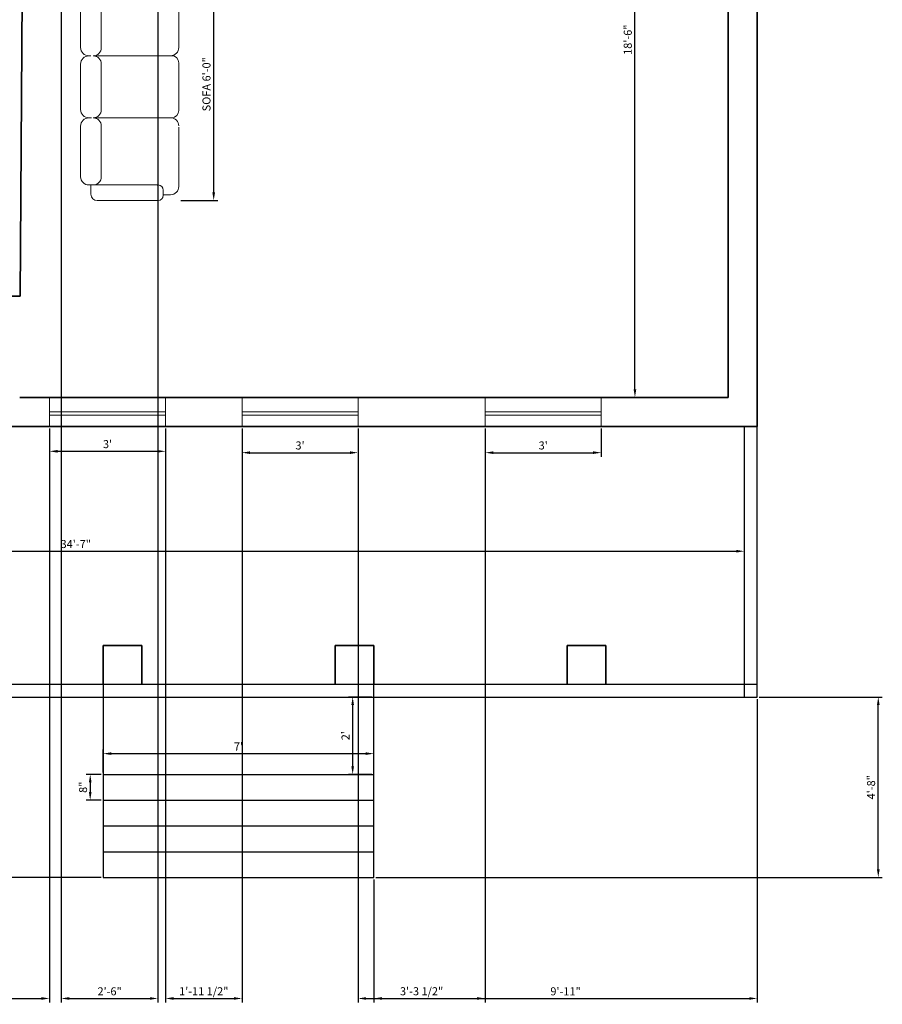
# Model space of a CAD drawing. Units: inches. Extents: x 2025 to 2528, y 1525 to 2336.
# Tile 4 of 18: x 2260 to 2528, y 1525 to 1831. Entities that reach past the tile are written whole.
import ezdxf

# ---------------------------------------------------------------- set-up
doc = ezdxf.new("R2010")
doc.units = ezdxf.units.IN
for name, color, linetype, lineweight in [('A-ANNO-DIMS', 2, 'Continuous', 18), ('A-COLS', 7, 'Continuous', 35), ('A-FLOR', 7, 'Continuous', 25), ('A-FLOR-STRS', 7, 'Continuous', 25), ('A-FURN', 8, 'Continuous', 18), ('A-GLAZ', 4, 'Continuous', 18), ('A-WALL', 7, 'Continuous', 35)]:
    doc.layers.add(name, color=color, linetype=linetype, lineweight=lineweight)
doc.styles.get("Standard").update_dxf_attribs({"font": 'arial.ttf'})
doc.dimstyles.new('Copy of ISO-25', dxfattribs={"dimtxt": 2.5, "dimasz": 2.5, "dimexe": 1.25, "dimexo": 0.625, "dimtad": 1, "dimdec": 1, "dimlunit": 4, "dimtxsty": 'Standard', "dimcen": 2.5, "dimadec": 0, "dimazin": 0, "dimtfac": 1, "dimtdec": 1, "dimtmove": 0, "dimatfit": 3, "dimfxl": 1, "dimarcsym": 0})

# ---------------------------------------------------------------- blocks, each defined once
blk = doc.blocks.new('*D31')
at = {"layer": 'A-ANNO-DIMS', "color": 0, "lineweight": -2, "transparency": 16777216}
for p, q in [((2479.39, 1935.41), (2449.8, 1935.41)), ((2451.05, 1715.91), (2451.05, 1932.91)), ((2479.39, 1713.41), (2449.8, 1713.41))]:
    blk.add_line(p, q, dxfattribs=at)
at = {"layer": 'A-ANNO-DIMS', "color": 0, "transparency": 16777216}
for points in [[(2450.63, 1932.91), (2451.46, 1932.91), (2451.05, 1935.41)], [(2450.63, 1715.91), (2451.46, 1715.91), (2451.05, 1713.41)]]:
    blk.add_solid(points, dxfattribs=at)
at = {"layer": 'Defpoints', "color": 0, "transparency": 16777216}
for p in [(2451.05, 1935.41), (2480.01, 1935.41), (2480.01, 1713.41)]:
    blk.add_point(p, dxfattribs=at)
at = {"layer": 'A-ANNO-DIMS', "color": 0, "transparency": 16777216, "insert": (2449.15, 1824.41), "char_height": 2.5, "attachment_point": 5, "rotation": 90}
blk.add_mtext('18\'-6"', dxfattribs=at)
blk = doc.blocks.new('*D37')
at = {"layer": 'A-ANNO-DIMS', "color": 0, "lineweight": -2, "transparency": 16777216}
for p, q in [((2269.37, 1703.79), (2269.37, 1695.43)), ((2305.37, 1703.79), (2305.37, 1695.43)), ((2271.87, 1696.68), (2302.87, 1696.68))]:
    blk.add_line(p, q, dxfattribs=at)
at = {"layer": 'A-ANNO-DIMS', "color": 0, "transparency": 16777216}
for points in [[(2271.87, 1697.09), (2271.87, 1696.26), (2269.37, 1696.68)], [(2302.87, 1697.09), (2302.87, 1696.26), (2305.37, 1696.68)]]:
    blk.add_solid(points, dxfattribs=at)
at = {"layer": 'Defpoints', "color": 0, "transparency": 16777216}
for p in [(2269.37, 1704.41), (2305.37, 1704.41), (2305.37, 1696.68)]:
    blk.add_point(p, dxfattribs=at)
at = {"layer": 'A-ANNO-DIMS', "color": 0, "transparency": 16777216, "insert": (2287.37, 1698.58), "char_height": 2.5, "attachment_point": 5}
blk.add_mtext("3'", dxfattribs=at)
blk = doc.blocks.new('*D38')
at = {"layer": 'A-ANNO-DIMS', "color": 0, "lineweight": -2, "transparency": 16777216}
for p, q in [((2329.1, 1703.79), (2329.1, 1695)), ((2365.1, 1703.79), (2365.1, 1695)), ((2331.6, 1696.25), (2362.6, 1696.25))]:
    blk.add_line(p, q, dxfattribs=at)
at = {"layer": 'A-ANNO-DIMS', "color": 0, "transparency": 16777216}
for points in [[(2331.6, 1696.67), (2331.6, 1695.84), (2329.1, 1696.25)], [(2362.6, 1696.67), (2362.6, 1695.84), (2365.1, 1696.25)]]:
    blk.add_solid(points, dxfattribs=at)
at = {"layer": 'Defpoints', "color": 0, "transparency": 16777216}
for p in [(2329.1, 1704.41), (2365.1, 1704.41), (2365.1, 1696.25)]:
    blk.add_point(p, dxfattribs=at)
at = {"layer": 'A-ANNO-DIMS', "color": 0, "transparency": 16777216, "insert": (2347.1, 1698.16), "char_height": 2.5, "attachment_point": 5}
blk.add_mtext("3'", dxfattribs=at)
blk = doc.blocks.new('*D39')
at = {"layer": 'A-ANNO-DIMS', "color": 0, "lineweight": -2, "transparency": 16777216}
for p, q in [((2404.58, 1703.79), (2404.58, 1695)), ((2440.58, 1703.79), (2440.58, 1695)), ((2407.08, 1696.25), (2438.08, 1696.25))]:
    blk.add_line(p, q, dxfattribs=at)
at = {"layer": 'A-ANNO-DIMS', "color": 0, "transparency": 16777216}
for points in [[(2407.08, 1696.67), (2407.08, 1695.84), (2404.58, 1696.25)], [(2438.08, 1696.67), (2438.08, 1695.84), (2440.58, 1696.25)]]:
    blk.add_solid(points, dxfattribs=at)
at = {"layer": 'Defpoints', "color": 0, "transparency": 16777216}
for p in [(2404.58, 1704.41), (2440.58, 1704.41), (2440.58, 1696.25)]:
    blk.add_point(p, dxfattribs=at)
at = {"layer": 'A-ANNO-DIMS', "color": 0, "transparency": 16777216, "insert": (2422.58, 1698.16), "char_height": 2.5, "attachment_point": 5}
blk.add_mtext("3'", dxfattribs=at)
blk = doc.blocks.new('*D40')
at = {"layer": 'A-ANNO-DIMS', "color": 0, "lineweight": -2, "transparency": 16777216}
for p, q in [((2070.01, 1625.04), (2070.01, 1666.92)), ((2072.51, 1665.67), (2482.51, 1665.67)), ((2485.01, 1625.04), (2485.01, 1666.92))]:
    blk.add_line(p, q, dxfattribs=at)
at = {"layer": 'A-ANNO-DIMS', "color": 0, "transparency": 16777216}
for points in [[(2072.51, 1666.08), (2072.51, 1665.25), (2070.01, 1665.67)], [(2482.51, 1666.08), (2482.51, 1665.25), (2485.01, 1665.67)]]:
    blk.add_solid(points, dxfattribs=at)
at = {"layer": 'Defpoints', "color": 0, "transparency": 16777216}
for p in [(2485.01, 1665.67), (2070.01, 1624.41), (2485.01, 1624.41)]:
    blk.add_point(p, dxfattribs=at)
at = {"layer": 'A-ANNO-DIMS', "color": 0, "transparency": 16777216, "insert": (2277.51, 1667.57), "char_height": 2.5, "attachment_point": 5}
blk.add_mtext('34\'-7"', dxfattribs=at)
blk = doc.blocks.new('*D41')
at = {"layer": 'A-ANNO-DIMS', "color": 0, "lineweight": -2, "transparency": 16777216}
for p, q in [((2286.01, 1597.04), (2286.01, 1604.1)), ((2288.51, 1602.85), (2367.51, 1602.85)), ((2370.01, 1597.04), (2370.01, 1604.1))]:
    blk.add_line(p, q, dxfattribs=at)
at = {"layer": 'A-ANNO-DIMS', "color": 0, "transparency": 16777216}
for points in [[(2288.51, 1603.27), (2288.51, 1602.44), (2286.01, 1602.85)], [(2367.51, 1603.27), (2367.51, 1602.44), (2370.01, 1602.85)]]:
    blk.add_solid(points, dxfattribs=at)
at = {"layer": 'Defpoints', "color": 0, "transparency": 16777216}
for p in [(2370.01, 1602.85), (2286.01, 1596.41), (2370.01, 1596.41)]:
    blk.add_point(p, dxfattribs=at)
at = {"layer": 'A-ANNO-DIMS', "color": 0, "transparency": 16777216, "insert": (2328.01, 1604.73), "char_height": 2.5, "attachment_point": 5}
blk.add_mtext("7'", dxfattribs=at)
blk = doc.blocks.new('*D42')
at = {"layer": 'A-ANNO-DIMS', "color": 0, "lineweight": -2, "transparency": 16777216}
for p, q in [((2369.39, 1620.41), (2362.19, 1620.41)), ((2363.44, 1617.91), (2363.44, 1598.91)), ((2369.39, 1596.41), (2362.19, 1596.41))]:
    blk.add_line(p, q, dxfattribs=at)
at = {"layer": 'A-ANNO-DIMS', "color": 0, "transparency": 16777216}
for points in [[(2363.02, 1617.91), (2363.86, 1617.91), (2363.44, 1620.41)], [(2363.02, 1598.91), (2363.86, 1598.91), (2363.44, 1596.41)]]:
    blk.add_solid(points, dxfattribs=at)
at = {"layer": 'Defpoints', "color": 0, "transparency": 16777216}
for p in [(2370.01, 1620.41), (2363.44, 1596.41), (2370.01, 1596.41)]:
    blk.add_point(p, dxfattribs=at)
at = {"layer": 'A-ANNO-DIMS', "color": 0, "transparency": 16777216, "insert": (2361.56, 1608.41), "char_height": 2.5, "attachment_point": 5, "rotation": 90}
blk.add_mtext("2'", dxfattribs=at)
blk = doc.blocks.new('*D43')
at = {"layer": 'A-ANNO-DIMS', "color": 0, "lineweight": -2, "transparency": 16777216}
for p, q in [((2285.39, 1596.41), (2280.74, 1596.41)), ((2281.99, 1593.91), (2281.99, 1590.91)), ((2285.39, 1588.41), (2280.74, 1588.41))]:
    blk.add_line(p, q, dxfattribs=at)
at = {"layer": 'A-ANNO-DIMS', "color": 0, "transparency": 16777216}
for points in [[(2281.58, 1593.91), (2282.41, 1593.91), (2281.99, 1596.41)], [(2281.58, 1590.91), (2282.41, 1590.91), (2281.99, 1588.41)]]:
    blk.add_solid(points, dxfattribs=at)
at = {"layer": 'Defpoints', "color": 0, "transparency": 16777216}
for p in [(2286.01, 1596.41), (2281.99, 1588.41), (2286.01, 1588.41)]:
    blk.add_point(p, dxfattribs=at)
at = {"layer": 'A-ANNO-DIMS', "color": 0, "transparency": 16777216, "insert": (2280.09, 1592.41), "char_height": 2.5, "attachment_point": 5, "rotation": 90}
blk.add_mtext('8"', dxfattribs=at)
blk = doc.blocks.new('A$C0876780F')
for p, q in [((0.15, 0.87), (0.15, 0.8444)), ((0.15, 0.87), (0.15, 0.85)), ((0.72, 0.95), (0.23, 0.95)), ((0.8, 0.85), (0.8, 0.87)), ((0.8, 0.87), (0.8, 0.85)), ((0.8, 0.87), (0.8, 0.8444)), ((1.32, 0.95), (0.88, 0.95)), ((1.4, 0.85), (1.4, 0.87)), ((1.4, 0.85), (1.4, 0.87)), ((1.48, 0.95), (2.02, 0.95)), ((2.1, 0.87), (2.1, 0.85)), ((2.1, 0.87), (2.1, 0.8444)), ((0, 0.79), (0, 0.21)), ((0.15, 0.85), (0.06, 0.85)), ((0.15, 0.21), (0.15, 0.85)), ((0.8011, 0.8204), (0.8011, 0.08)), ((1.4014, 0.08), (1.4014, 0.803)), ((2.1, 0.21), (2.1, 0.85)), ((2.1, 0.85), (2.19, 0.85)), ((2.25, 0.79), (2.25, 0.21)), ((0.72, 0.75), (0.23, 0.75)), ((1.32, 0.75), (0.88, 0.75)), ((1.48, 0.75), (2.02, 0.75)), ((0, 0.21), (0, 0.2)), ((0.15, 0.2), (0.15, 0.25)), ((2.1, 0.2), (2.1, 0.25)), ((2.25, 0.21), (2.25, 0.2)), ((0.05, 0.15), (0.1, 0.15)), ((0.056, 0.15), (0.056, 0.08)), ((2.2, 0.15), (2.15, 0.15)), ((2.194, 0.15), (2.194, 0.08)), ((0.136, 0), (0.7093, 0)), ((0.8011, 0.07), (0.8011, 0.08)), ((0.8711, 0), (1.3314, 0)), ((1.4014, 0.07), (1.4014, 0.08)), ((2.114, 0), (1.48, 0))]:
    blk.add_line(p, q)
for centre, radius, start, end in [((0.23, 0.87), 0.08, 90, 180), ((0.72, 0.87), 0.08, 0, 90), ((0.88, 0.87), 0.08, 90, 180), ((1.32, 0.87), 0.08, 0, 90), ((1.48, 0.87), 0.08, 90, 180), ((2.02, 0.87), 0.08, 0, 90), ((0.06, 0.79), 0.06, 90, 180), ((0.23, 0.83), 0.08, 180, 270), ((0.23, 0.83), 0.08, 180, 270), ((0.72, 0.83), 0.08, 270, 0), ((0.88, 0.83), 0.08, 180, 270), ((0.88, 0.83), 0.08, 180, 270), ((1.32, 0.83), 0.08, 270, 0), ((1.48, 0.83), 0.08, 180, 270), ((2.02, 0.83), 0.08, 270, 0), ((2.02, 0.83), 0.08, 270, 0), ((2.19, 0.79), 0.06, 0, 90), ((0.05, 0.2), 0.05, 180, 270), ((0.1, 0.2), 0.05, 270, 0), ((0.09, 0.21), 0.06, 350.53768, 0), ((2.16, 0.21), 0.06, 180, 189.46232), ((2.15, 0.2), 0.05, 180, 270), ((2.2, 0.2), 0.05, 270, 0), ((0.136, 0.08), 0.08, 180, 270), ((0.7211, 0.08), 0.08, 270, 0), ((0.8711, 0.07), 0.07, 180, 270), ((1.3314, 0.07), 0.07, 270, 0), ((1.4814, 0.08), 0.08, 180, 270), ((2.114, 0.08), 0.08, 270, 0)]:
    blk.add_arc(centre, radius, start, end)
blk = doc.blocks.new('WIN-36-PORCH')
for p, q in [((0, 0), (0, 9)), ((36, 9), (36, 0)), ((0, 4.5), (36, 4.5)), ((0, 3.5), (36, 3.5)), ((36, 0), (0, 0))]:
    blk.add_line(p, q)
blk = doc.blocks.new('POST-PORCH-12')
for p, q in [((12, 12), (0, 12)), ((12, 0), (12, 12)), ((0, 0), (12, 0))]:
    blk.add_line(p, q)
blk = doc.blocks.new('*D58')
at = {"layer": 'A-ANNO-DIMS', "color": 0, "lineweight": -2, "transparency": 16777216}
for p, q in [((2310.12, 1846.66), (2321.57, 1846.66)), ((2320.32, 1777.01), (2320.32, 1844.16)), ((2310.12, 1774.51), (2321.57, 1774.51))]:
    blk.add_line(p, q, dxfattribs=at)
at = {"layer": 'A-ANNO-DIMS', "color": 0, "transparency": 16777216}
for points in [[(2319.9, 1844.16), (2320.73, 1844.16), (2320.32, 1846.66)], [(2319.9, 1777.01), (2320.73, 1777.01), (2320.32, 1774.51)]]:
    blk.add_solid(points, dxfattribs=at)
at = {"layer": 'Defpoints', "color": 0, "transparency": 16777216}
for p in [(2309.49, 1846.66), (2320.32, 1846.66), (2309.49, 1774.51)]:
    blk.add_point(p, dxfattribs=at)
at = {"layer": 'A-ANNO-DIMS', "color": 0, "transparency": 16777216, "insert": (2318.4, 1810.58), "char_height": 2.5, "attachment_point": 5, "rotation": 90}
blk.add_mtext('SOFA 6\'-0"', dxfattribs=at)
blk = doc.blocks.new('*D67')
at = {"layer": 'A-ANNO-DIMS', "color": 0, "lineweight": -2, "transparency": 16777216}
for p, q in [((2207.01, 1703.79), (2207.01, 1525.61)), ((2269.37, 1703.79), (2269.37, 1525.61)), ((2209.51, 1526.86), (2266.87, 1526.86))]:
    blk.add_line(p, q, dxfattribs=at)
at = {"layer": 'A-ANNO-DIMS', "color": 0, "transparency": 16777216}
for points in [[(2209.51, 1527.28), (2209.51, 1526.45), (2207.01, 1526.86)], [(2266.87, 1527.28), (2266.87, 1526.45), (2269.37, 1526.86)]]:
    blk.add_solid(points, dxfattribs=at)
at = {"layer": 'Defpoints', "color": 0, "transparency": 16777216}
for p in [(2207.01, 1704.41), (2269.37, 1704.41), (2269.37, 1526.86)]:
    blk.add_point(p, dxfattribs=at)
at = {"layer": 'A-ANNO-DIMS', "color": 0, "transparency": 16777216, "insert": (2238.19, 1528.78), "char_height": 2.5, "attachment_point": 5}
blk.add_mtext('5\'-2 1/2"', dxfattribs=at)
blk = doc.blocks.new('*D68')
at = {"layer": 'A-ANNO-DIMS', "color": 0, "lineweight": -2, "transparency": 16777216}
for p, q in [((2305.37, 1703.79), (2305.37, 1525.61)), ((2329.1, 1703.79), (2329.1, 1525.61)), ((2307.87, 1526.86), (2326.6, 1526.86))]:
    blk.add_line(p, q, dxfattribs=at)
at = {"layer": 'A-ANNO-DIMS', "color": 0, "transparency": 16777216}
for points in [[(2307.87, 1527.28), (2307.87, 1526.45), (2305.37, 1526.86)], [(2326.6, 1527.28), (2326.6, 1526.45), (2329.1, 1526.86)]]:
    blk.add_solid(points, dxfattribs=at)
at = {"layer": 'Defpoints', "color": 0, "transparency": 16777216}
for p in [(2305.37, 1704.41), (2329.1, 1704.41), (2329.1, 1526.86)]:
    blk.add_point(p, dxfattribs=at)
at = {"layer": 'A-ANNO-DIMS', "color": 0, "transparency": 16777216, "insert": (2317.23, 1528.78), "char_height": 2.5, "attachment_point": 5}
blk.add_mtext('1\'-11 1/2"', dxfattribs=at)
blk = doc.blocks.new('*D69')
at = {"layer": 'A-ANNO-DIMS', "color": 0, "lineweight": -2, "transparency": 16777216}
for p, q in [((2365.1, 1703.79), (2365.1, 1525.61)), ((2404.58, 1703.79), (2404.58, 1525.61)), ((2367.6, 1526.86), (2402.08, 1526.86))]:
    blk.add_line(p, q, dxfattribs=at)
at = {"layer": 'A-ANNO-DIMS', "color": 0, "transparency": 16777216}
for points in [[(2367.6, 1527.28), (2367.6, 1526.45), (2365.1, 1526.86)], [(2402.08, 1527.28), (2402.08, 1526.45), (2404.58, 1526.86)]]:
    blk.add_solid(points, dxfattribs=at)
at = {"layer": 'Defpoints', "color": 0, "transparency": 16777216}
for p in [(2365.1, 1704.41), (2404.58, 1704.41), (2404.58, 1526.86)]:
    blk.add_point(p, dxfattribs=at)
at = {"layer": 'A-ANNO-DIMS', "color": 0, "transparency": 16777216, "insert": (2384.84, 1528.78), "char_height": 2.5, "attachment_point": 5}
blk.add_mtext('3\'-3 1/2"', dxfattribs=at)
blk = doc.blocks.new('*D71')
at = {"layer": 'A-ANNO-DIMS', "color": 0, "lineweight": -2, "transparency": 16777216}
for p, q in [((2489.01, 1619.79), (2489.01, 1525.61)), ((2370.01, 1563.79), (2370.01, 1525.61)), ((2372.51, 1526.86), (2486.51, 1526.86))]:
    blk.add_line(p, q, dxfattribs=at)
at = {"layer": 'A-ANNO-DIMS', "color": 0, "transparency": 16777216}
for points in [[(2372.51, 1527.28), (2372.51, 1526.45), (2370.01, 1526.86)], [(2486.51, 1527.28), (2486.51, 1526.45), (2489.01, 1526.86)]]:
    blk.add_solid(points, dxfattribs=at)
at = {"layer": 'Defpoints', "color": 0, "transparency": 16777216}
for p in [(2489.01, 1620.41), (2370.01, 1564.41), (2489.01, 1526.86)]:
    blk.add_point(p, dxfattribs=at)
at = {"layer": 'A-ANNO-DIMS', "color": 0, "transparency": 16777216, "insert": (2429.51, 1528.76), "char_height": 2.5, "attachment_point": 5}
blk.add_mtext('9\'-11"', dxfattribs=at)
blk = doc.blocks.new('*D72')
at = {"layer": 'A-ANNO-DIMS', "color": 0, "lineweight": -2, "transparency": 16777216}
for p, q in [((2489.64, 1620.41), (2527.81, 1620.41)), ((2526.56, 1566.91), (2526.56, 1617.91)), ((2370.64, 1564.41), (2527.81, 1564.41))]:
    blk.add_line(p, q, dxfattribs=at)
at = {"layer": 'A-ANNO-DIMS', "color": 0, "transparency": 16777216}
for points in [[(2526.15, 1617.91), (2526.98, 1617.91), (2526.56, 1620.41)], [(2526.15, 1566.91), (2526.98, 1566.91), (2526.56, 1564.41)]]:
    blk.add_solid(points, dxfattribs=at)
at = {"layer": 'Defpoints', "color": 0, "transparency": 16777216}
for p in [(2489.01, 1620.41), (2526.56, 1620.41), (2370.01, 1564.41)]:
    blk.add_point(p, dxfattribs=at)
at = {"layer": 'A-ANNO-DIMS', "color": 0, "transparency": 16777216, "insert": (2524.66, 1592.41), "char_height": 2.5, "attachment_point": 5, "rotation": 90}
blk.add_mtext('4\'-8"', dxfattribs=at)
blk = doc.blocks.new('*D76')
at = {"layer": 'A-ANNO-DIMS', "color": 0, "lineweight": -2, "transparency": 16777216}
for p, q in [((2273.01, 2114.79), (2273.01, 1525.61)), ((2303.01, 2114.79), (2303.01, 1525.61)), ((2275.51, 1526.86), (2300.51, 1526.86))]:
    blk.add_line(p, q, dxfattribs=at)
at = {"layer": 'A-ANNO-DIMS', "color": 0, "transparency": 16777216}
for points in [[(2275.51, 1527.28), (2275.51, 1526.45), (2273.01, 1526.86)], [(2300.51, 1527.28), (2300.51, 1526.45), (2303.01, 1526.86)]]:
    blk.add_solid(points, dxfattribs=at)
at = {"layer": 'Defpoints', "color": 0, "transparency": 16777216}
for p in [(2273.01, 2115.41), (2303.01, 2115.41), (2303.01, 1526.86)]:
    blk.add_point(p, dxfattribs=at)
at = {"layer": 'A-ANNO-DIMS', "color": 0, "transparency": 16777216, "insert": (2288.01, 1528.76), "char_height": 2.5, "attachment_point": 5}
blk.add_mtext('2\'-6"', dxfattribs=at)
blk = doc.blocks.new('*D80')
at = {"layer": 'A-ANNO-DIMS', "color": 0, "lineweight": -2, "transparency": 16777216}
for p, q in [((2065.39, 2292.41), (2027.21, 2292.41)), ((2028.46, 1566.91), (2028.46, 2289.91)), ((2285.39, 1564.41), (2027.21, 1564.41))]:
    blk.add_line(p, q, dxfattribs=at)
at = {"layer": 'A-ANNO-DIMS', "color": 0, "transparency": 16777216}
for points in [[(2028.05, 2289.91), (2028.88, 2289.91), (2028.46, 2292.41)], [(2028.05, 1566.91), (2028.88, 1566.91), (2028.46, 1564.41)]]:
    blk.add_solid(points, dxfattribs=at)
at = {"layer": 'Defpoints', "color": 0, "transparency": 16777216}
for p in [(2028.46, 2292.41), (2066.01, 2292.41), (2286.01, 1564.41)]:
    blk.add_point(p, dxfattribs=at)
at = {"layer": 'A-ANNO-DIMS', "color": 0, "transparency": 16777216, "insert": (2026.56, 1928.41), "char_height": 2.5, "attachment_point": 5, "rotation": 90}
blk.add_mtext('60\'-8"', dxfattribs=at)

msp = doc.modelspace()

# ---------------------------------------------------------------- linework, layer by layer
at = {"layer": 'A-FLOR'}
for p, q in [((2485.01, 1620.41), (2485.01, 1704.41)), ((2489.01, 1620.41), (2489.01, 1704.41)), ((2066.01, 1624.41), (2489.01, 1624.41)), ((2226.01, 1624.41), (2286.01, 1624.41)), ((2298.01, 1624.41), (2358.01, 1624.41)), ((2370.01, 1624.41), (2430.01, 1624.41)), ((2066.01, 1620.41), (2489.01, 1620.41))]:
    msp.add_line(p, q, dxfattribs=at)
at = {"layer": 'A-FLOR-STRS'}
for p, q in [((2286.01, 1624.41), (2286.01, 1620.41)), ((2370.01, 1596.41), (2370.01, 1624.41)), ((2286.01, 1620.41), (2286.01, 1596.41)), ((2286.01, 1596.41), (2370.01, 1596.41)), ((2286.01, 1596.41), (2286.01, 1588.41)), ((2370.01, 1588.41), (2370.01, 1596.41)), ((2286.01, 1588.41), (2370.01, 1588.41)), ((2286.01, 1588.41), (2286.01, 1580.41)), ((2370.01, 1580.41), (2370.01, 1588.41)), ((2286.01, 1580.41), (2370.01, 1580.41)), ((2286.01, 1580.41), (2286.01, 1572.41)), ((2370.01, 1572.41), (2370.01, 1580.41)), ((2286.01, 1572.41), (2370.01, 1572.41)), ((2286.01, 1572.41), (2286.01, 1564.41)), ((2370.01, 1564.41), (2370.01, 1572.41)), ((2286.01, 1564.41), (2370.01, 1564.41))]:
    msp.add_line(p, q, dxfattribs=at)
at = {"layer": 'A-WALL'}
for p, q in [((2489.01, 1704.41), (2489.01, 2283.41)), ((2480.01, 1713.41), (2480.01, 2195.22)), ((2260.29, 1744.82), (2261.01, 1869.41)), ((2254.35, 1744.85), (2260.29, 1744.82)), ((2260.11, 1713.41), (2260.11, 1713.41)), ((2260.11, 1713.41), (2269.37, 1713.41)), ((2260.11, 1713.41), (2480.01, 1713.41)), ((2315.01, 1713.41), (2309.01, 1713.41)), ((2404.57, 1713.41), (2365.1, 1713.41)), ((2480.01, 1713.41), (2440.58, 1713.41)), ((2066.01, 1704.41), (2489.01, 1704.41))]:
    msp.add_line(p, q, dxfattribs=at)

# ---------------------------------------------------------------- block references
at = {"layer": 'A-COLS', "rotation": 90}
for p in [(2298.01, 1624.41), (2370.01, 1624.41), (2442.01, 1624.41)]:
    msp.add_blockref('POST-PORCH-12', p, dxfattribs=at)
at = {"layer": 'A-FURN', "xscale": 32.06799314308715, "yscale": 32.06799314308715, "zscale": 32.06799314308715, "rotation": 90}
msp.add_blockref('A$C0876780F', (2309.49, 1774.51), dxfattribs=at)
at = {"layer": 'A-GLAZ'}
for p in [(2269.37, 1704.41), (2329.1, 1704.41), (2404.57, 1704.41)]:
    msp.add_blockref('WIN-36-PORCH', p, dxfattribs=at)

# ---------------------------------------------------------------- dimensions: what is measured, and where the dimension line sits
at = {"layer": 'A-ANNO-DIMS'}
for base, p1, p2, override, picture, middle in [((2028.46, 2292.41), (2286.01, 1564.41), (2066.01, 2292.41), {"dimdec": 1, "dimlfac": 1, "dimrnd": 0, "dimzin": 1, "dimdsep": 46, "dimlunit": 4, "dimfrac": 2}, '*D80', (2026.56, 1928.41)), ((2451.05, 1935.41), (2480.01, 1713.41), (2480.01, 1935.41), {"dimclrd": 0, "dimclre": 0, "dimclrt": 0}, '*D31', (2449.15, 1824.41)), ((2363.44, 1596.41), (2370.01, 1620.41), (2370.01, 1596.41), {"dimclrd": 0, "dimclre": 0, "dimclrt": 0}, '*D42', (2361.56, 1608.41)), ((2526.56, 1620.41), (2370.01, 1564.41), (2489.01, 1620.41), {"dimdec": 1, "dimlfac": 1, "dimrnd": 0, "dimzin": 1, "dimdsep": 46, "dimlunit": 4, "dimfrac": 2}, '*D72', (2524.66, 1592.41)), ((2281.99, 1588.41), (2286.01, 1596.41), (2286.01, 1588.41), {"dimclrd": 0, "dimclre": 0, "dimclrt": 0}, '*D43', (2280.09, 1592.41))]:
    dim = msp.add_linear_dim(base=base, p1=p1, p2=p2, angle=90, dimstyle='Copy of ISO-25', override=override, dxfattribs=at)
    dim.commit()
    dim.dimension.update_dxf_attribs({"geometry": picture, "text_midpoint": middle})
for base, p1, p2, override, picture, middle in [((2303.01, 1526.86), (2273.01, 2115.41), (2303.01, 2115.41), {"dimdec": 1, "dimlfac": 1, "dimrnd": 0, "dimzin": 1, "dimdsep": 46, "dimlunit": 4, "dimfrac": 2}, '*D76', (2288.01, 1528.76)), ((2269.37, 1526.86), (2207.01, 1704.41), (2269.37, 1704.41), {"dimdec": 1, "dimlfac": 1, "dimrnd": 0, "dimzin": 1, "dimdsep": 46, "dimlunit": 4, "dimfrac": 2}, '*D67', (2238.19, 1528.78)), ((2305.37, 1696.68), (2269.37, 1704.41), (2305.37, 1704.41), {"dimclrd": 0, "dimclre": 0, "dimclrt": 0}, '*D37', (2287.37, 1698.58)), ((2329.1, 1526.86), (2305.37, 1704.41), (2329.1, 1704.41), {"dimdec": 1, "dimlfac": 1, "dimrnd": 0, "dimzin": 1, "dimdsep": 46, "dimlunit": 4, "dimfrac": 2}, '*D68', (2317.23, 1528.78)), ((2365.1, 1696.25), (2329.1, 1704.41), (2365.1, 1704.41), {"dimclrd": 0, "dimclre": 0, "dimclrt": 0}, '*D38', (2347.1, 1698.16)), ((2404.57, 1526.86), (2365.1, 1704.41), (2404.57, 1704.41), {"dimdec": 1, "dimlfac": 1, "dimrnd": 0, "dimzin": 1, "dimdsep": 46, "dimlunit": 4, "dimfrac": 2}, '*D69', (2384.84, 1528.78)), ((2440.58, 1696.25), (2404.57, 1704.41), (2440.58, 1704.41), {"dimclrd": 0, "dimclre": 0, "dimclrt": 0}, '*D39', (2422.58, 1698.16)), ((2485.01, 1665.67), (2070.01, 1624.41), (2485.01, 1624.41), {"dimclrd": 0, "dimclre": 0, "dimclrt": 0}, '*D40', (2277.51, 1667.57)), ((2489.01, 1526.86), (2370.01, 1564.41), (2489.01, 1620.41), {"dimdec": 1, "dimlfac": 1, "dimrnd": 0, "dimzin": 1, "dimdsep": 46, "dimlunit": 4, "dimfrac": 2}, '*D71', (2429.51, 1528.76)), ((2370.01, 1602.85), (2286.01, 1596.41), (2370.01, 1596.41), {"dimclrd": 0, "dimclre": 0, "dimclrt": 0}, '*D41', (2328.01, 1604.73))]:
    dim = msp.add_linear_dim(base=base, p1=p1, p2=p2, dimstyle='Copy of ISO-25', override=override, dxfattribs=at)
    dim.commit()
    dim.dimension.update_dxf_attribs({"geometry": picture, "text_midpoint": middle})
dim = msp.add_linear_dim(base=(2320.3169, 1846.6606), p1=(2309.494, 1774.5076), p2=(2309.494, 1846.6606), angle=90, text='SOFA <>', dimstyle='Copy of ISO-25', override={"dimdec": 1, "dimlfac": 1, "dimrnd": 0, "dimzin": 1, "dimdsep": 46, "dimlunit": 4, "dimfrac": 2}, dxfattribs=at)
dim.commit()
dim.dimension.update_dxf_attribs({"geometry": '*D58', "text_midpoint": (2318.3984, 1810.5841)})

doc.saveas('drawing.dxf')
